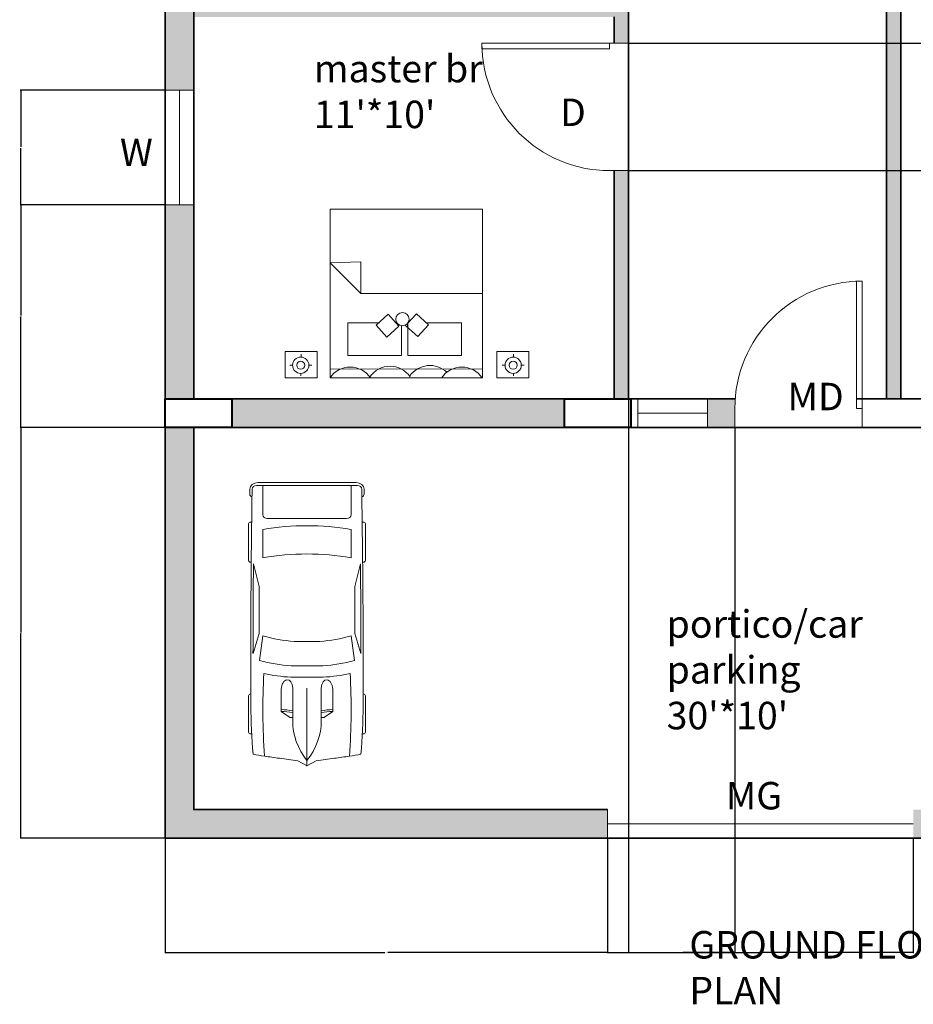
# Model space of a CAD drawing. Units: inches. Extents: x 1568 to 2529, y 2149 to 2897.
# Tile 1 of 16: x 1568 to 1849, y 2149 to 2459. Entities that reach past the tile are written whole.
import ezdxf

# ---------------------------------------------------------------- set-up
doc = ezdxf.new("R2010")
doc.units = ezdxf.units.IN
for name, color, linetype, lineweight in [('A-ANNO-DIMS', 2, 'Continuous', 18), ('A-AREA-IDEN', 210, 'Continuous', 18), ('A-COLS', 7, 'Continuous', 40), ('A-DOOR', 4, 'Continuous', 18), ('A-FURN', 8, 'Continuous', 18), ('A-WALL-PATT', 172, 'Continuous', 13), ('C-PKNG-VEHI', 8, 'Continuous', 13), ('text', 210, 'Continuous', 18), ('wall', 7, 'Continuous', 35), ('window', 130, 'Continuous', 18)]:
    doc.layers.add(name, color=color, linetype=linetype, lineweight=lineweight)
doc.styles.get("Standard").update_dxf_attribs({"font": 'arial.ttf'})
doc.dimstyles.get("Standard").update_dxf_attribs({"dimtxt": 0.18, "dimasz": 0.18, "dimexe": 0.18, "dimexo": 0.0625, "dimgap": 0.09, "dimtad": 0, "dimtih": 1, "dimtoh": 1, "dimdec": 4, "dimzin": 0, "dimdsep": 46, "dimtxsty": 'Standard', "dimcen": 0.09, "dimadec": 0, "dimazin": 0, "dimtfac": 1, "dimtdec": 4, "dimtofl": 0, "dimtmove": 0, "dimatfit": 3, "dimfxl": 1, "dimtolj": 1, "dimtzin": 0, "dimarcsym": 0})

# ---------------------------------------------------------------- blocks, each defined once
blk = doc.blocks.new('*U2')
for p, q in [((0, 0), (0, -6)), ((40, 0), (40, -6))]:
    blk.add_line(p, q)
blk.add_lwpolyline([(0, 0), (0, 40), (1.75, 40), (1.75, 0)], close=True)
blk.add_arc((0, 0), 40, 0, 90)
blk = doc.blocks.new('*U8')
for p, q in [((21.1, 37.41), (21.1, 36.83)), ((46.55, 38.89), (22.35, 38.89)), ((47.8, 37.39), (47.8, 37.41)), ((87.99, 31.87), (74.76, 35.92)), ((134.31, 35.6), (119.29, 31.78)), ((135.45, 37.07), (135.45, 37.41)), ((136.7, 38.89), (160.9, 38.89)), ((162.15, 37.41), (162.15, 36.77)), ((186.47, -33.5), (186.47, 33.5)), ((70.03, 31.54), (86.41, 29.35)), ((138.42, 29.35), (157.25, 29.35)), ((164.52, 26.39), (164.52, -26.39)), ((186.47, 29.35), (167.01, 29.35)), ((188.4, -32.76), (188.4, 32.76)), ((32.27, 11.63), (36.13, 17.17)), ((36.13, 17.17), (50.94, 17.17)), ((29.77, 9.51), (51.68, 9.51)), ((32.12, 9.51), (32.12, 11.15)), ((58.92, -10.77), (58.92, 10.77)), ((66.55, -10.53), (66.55, 10.53)), ((82.74, 8.5), (82.74, -8.5)), ((186.47, -10.53), (186.47, 10.53)), ((3.27, 6.13), (0.1, 0.41)), ((0, 0), (51.68, 0)), ((0.1, -0.41), (3.27, -6.13)), ((29.77, -9.51), (51.68, -9.51)), ((32.12, -9.51), (32.12, -11.15)), ((32.27, -11.63), (36.13, -17.17)), ((36.13, -17.17), (50.94, -17.17)), ((86.41, -29.35), (70.03, -31.54)), ((87.99, -31.87), (74.76, -35.92)), ((134.31, -35.6), (119.29, -31.78)), ((157.25, -29.35), (138.42, -29.35)), ((167.01, -29.35), (186.47, -29.35)), ((21.1, -37.41), (21.1, -36.83)), ((46.55, -38.89), (22.35, -38.89)), ((47.8, -37.39), (47.8, -37.41)), ((135.45, -37.07), (135.45, -37.41)), ((136.7, -38.89), (160.9, -38.89)), ((162.15, -37.41), (162.15, -36.77))]:
    blk.add_line(p, q)
for centre, major_axis, ratio, start_param, end_param in [((266.03, -27.52), (0, 313.31), 0.842304, 1.367076, 1.39176), ((41.19, -490.86), (0, 528.23), 0.842304, 0.00281, 0.075598), ((22.35, 37.41), (0, -1.48), 0.842304, 3.141593, 4.712389), ((64.48, -10555.62), (0, 10593.03), 0.842304, -0.013397, 0.002797), ((46.55, 37.41), (0, 1.48), 0.842304, -1.570796, 0), ((64.48, -10555.62), (0, -10591.55), 0.842304, 3.133765, 3.140441), ((136.7, 37.41), (0, -1.48), 0.842304, 3.141593, 4.712389), ((160.9, 37.41), (0, 1.48), 0.842304, -1.570796, 0), ((180.63, 35.84), (0, 2.22), 0.842304, -0.013017, 1.249894), ((64.48, -10556.36), (0, 10595.31), 0.842304, -0.013397, -0.013017), ((183.98, 33.5), (0, -2.96), 0.842304, 1.570796, 3.128196), ((183.98, 32.76), (0, -5.25), 0.842304, 1.570796, 3.128196), ((259.18, -27.52), (0, -305.3), 0.842304, 4.528606, 4.561838), ((37.47, -593.96), (0, -623.33), 0.842304, 3.096046, 3.200911), ((134.4, 5.39), (0, -89.78), 0.842304, 4.449482, 4.652344), ((135.29, 5.39), (0, 81.77), 0.842304, 1.245306, 1.50788), ((149.6, 2.8), (0, -79.58), 0.842304, 4.372215, 4.640744), ((95.79, -3666.35), (0, -3698.24), 0.842304, 3.134049, 3.144098), ((17.08, 0), (0, 147.02), 0.842304, 4.511394, 4.913384), ((35.91, 0), (0, 147.02), 0.842304, 4.511394, 4.913384), ((167.01, 26.39), (0, 2.96), 0.842304, 0, 1.570796), ((-204.49, 52.4), (0, -250.96), 0.842304, 1.385369, 1.434372), ((13.04, 17.01), (0, 27.42), 0.842304, 4.435146, 4.718221), ((14.2, 17.01), (0, 27.42), 0.842304, 4.435146, 4.718221), ((50.79, 13.34), (6.34, -0.36), 0.603834, -1.395552, 1.581315), ((29.77, -46.66), (0, 56.17), 0.842304, 0, 0.590319), ((32.75, 11.15), (0, 0.74), 0.842304, 0.879714, 1.570796), ((0.62, 0), (0, -0.74), 0.842304, 4.131459, 5.293319), ((-204.49, -52.4), (0, 250.96), 0.842304, -1.434372, -1.385369), ((29.77, 46.66), (0, 56.17), 0.842304, 2.551274, 3.141593), ((32.75, -11.15), (0, -0.74), 0.842304, 4.712389, 5.403472), ((13.04, -17.01), (0, -27.42), 0.842304, 1.564964, 1.848039), ((14.2, -17.01), (0, -27.42), 0.842304, 1.564964, 1.848039), ((134.4, -5.39), (0, -89.78), 0.842304, -1.510751, -1.307889), ((135.29, -5.39), (0, -81.77), 0.842304, -1.50788, -1.245306), ((149.6, -2.8), (0, -79.58), 0.842304, -1.499151, -1.230623), ((259.18, 27.52), (0, 305.3), 0.842304, 1.721348, 1.754579), ((266.03, 27.52), (0, 313.31), 0.842304, 1.749832, 1.774517), ((37.47, 593.96), (0, -623.33), 0.842304, -0.059319, 0.045547), ((95.79, 3666.35), (0, -3698.24), 0.842304, -0.002505, 0.007544), ((167.01, -26.39), (0, -2.96), 0.842304, 4.712389, 6.283185), ((183.98, -32.76), (0, -5.25), 0.842304, 0.013397, 1.570796), ((41.19, 490.86), (0, -528.23), 0.842304, -0.075598, -0.00281), ((22.35, -37.41), (0, 1.48), 0.842304, 1.570796, 3.141593), ((64.48, 10555.62), (0, 10593.03), 0.842304, 3.138796, 3.15499), ((46.55, -37.41), (0, -1.48), 0.842304, 0, 1.570796), ((64.48, 10555.62), (0, -10591.55), 0.842304, 0.001152, 0.007828), ((136.7, -37.41), (0, -1.48), 0.842304, -1.570796, 0), ((160.9, -37.41), (0, 1.48), 0.842304, 3.141593, 4.712389), ((180.63, -35.84), (0, -2.22), 0.842304, -1.249894, 0.013017), ((64.48, 10556.36), (0, 10595.31), 0.842304, 3.15461, 3.15499), ((183.98, -33.5), (0, 2.96), 0.842304, 3.15499, 4.712389)]:
    blk.add_ellipse(centre, major_axis=major_axis, ratio=ratio, start_param=start_param, end_param=end_param)
at = {"extrusion": (0, 0, -1)}
blk.add_ellipse((50.79, -13.34), major_axis=(6.34, 0.36), ratio=0.603834, start_param=-1.395552, end_param=1.581315, dxfattribs=at)
blk = doc.blocks.new('BED-WITH-NIGHTSTANDS')
for p, q in [((14.05, 36.12), (23.68, 36.4)), ((23.68, 26.45), (14.05, 36.12)), ((23.68, 36.4), (23.68, 26.45)), ((61.95, 26.45), (23.68, 26.45)), ((38.01, 16.14), (37.63, 16.49)), ((38.35, 15.84), (38.01, 16.14)), ((38.35, 16.98), (38.35, 15.84)), ((5, 6.48), (5, 7.42)), ((71.71, 6.48), (71.71, 7.42)), ((2.29, 3.95), (1.38, 3.95)), ((7.42, 3.92), (8.29, 3.92)), ((69, 3.95), (68.1, 3.95)), ((74.13, 3.92), (75, 3.92)), ((4.92, 1.35), (4.92, 0.55)), ((14.05, 2.79), (61.95, 2.73)), ((71.64, 1.35), (71.64, 0.55))]:
    blk.add_line(p, q)
for points in [[(14.05, 0), (61.95, 0), (61.95, 52.9), (14.05, 52.9)], [(31.9, 12.77), (35.7, 16.21), (32.32, 19.94), (28.52, 16.5)], [(10.04, 0), (0, 0), (0, 8.21), (10.04, 8.21)], [(76.49, 0), (66.44, 0), (66.44, 8.21), (76.49, 8.21)]]:
    blk.add_lwpolyline(points, close=True)
for points in [[(38.35, 16.98), (41.16, 20.08), (44.96, 16.64), (41.58, 12.91), (38.01, 16.14)], [(29.36, 17.26), (19.65, 17.26), (19.65, 6.93), (36.45, 6.93), (36.45, 16.34)], [(35.04, 17.26), (34.75, 17.26)], [(38.52, 17.23), (38.52, 6.93), (55.32, 6.93), (55.32, 17.26), (44.28, 17.26)], [(38.6, 17.26), (38.54, 17.26)]]:
    blk.add_lwpolyline(points)
for centre, radius in [((36.79, 18.4), 2.09), ((4.85, 3.92), 2.56), ((71.57, 3.92), 2.56), ((4.85, 3.92), 1.27), ((71.57, 3.92), 1.27)]:
    blk.add_circle(centre, radius)
for centre, start in [((20.4, -4.37), 34.5304), ((32.9, -4.09), 34.5304), ((45.42, -3.86), 46.3255), ((55.47, -4.37), 34.5304)]:
    blk.add_arc(centre, 7.71, start, 145.4696)
blk = doc.blocks.new('*D29')
at = {"layer": 'A-ANNO-DIMS', "color": 0, "lineweight": -2, "transparency": 16777216}
for p, q in [((1613.49, 2330.53), (1567.99, 2330.53)), ((1568.17, 2330.35), (1568.17, 2266.21)), ((1568.17, 2201.71), (1568.17, 2265.85)), ((1613.49, 2201.53), (1567.99, 2201.53))]:
    blk.add_line(p, q, dxfattribs=at)
at = {"layer": 'A-ANNO-DIMS', "color": 0, "transparency": 16777216}
for points in [[(1568.14, 2330.35), (1568.2, 2330.35), (1568.17, 2330.53)], [(1568.14, 2201.71), (1568.2, 2201.71), (1568.17, 2201.53)]]:
    blk.add_solid(points, dxfattribs=at)
at = {"layer": 'Defpoints', "color": 0, "transparency": 16777216}
for p in [(1568.17, 2330.53), (1613.55, 2330.53), (1613.55, 2201.53)]:
    blk.add_point(p, dxfattribs=at)
at = {"layer": 'A-ANNO-DIMS', "color": 0, "transparency": 16777216, "insert": (1568.17, 2266.03), "char_height": 0.18, "attachment_point": 5}
blk.add_mtext('\\A1;129', dxfattribs=at)
blk = doc.blocks.new('*D30')
at = {"layer": 'A-ANNO-DIMS', "color": 0, "lineweight": -2, "transparency": 16777216}
for p, q in [((1613.55, 2201.47), (1613.55, 2165.5)), ((1752.52, 2201.47), (1752.52, 2165.5)), ((1613.73, 2165.68), (1682.58, 2165.68)), ((1752.34, 2165.68), (1683.49, 2165.68))]:
    blk.add_line(p, q, dxfattribs=at)
at = {"layer": 'A-ANNO-DIMS', "color": 0, "transparency": 16777216}
for points in [[(1613.73, 2165.71), (1613.73, 2165.65), (1613.55, 2165.68)], [(1752.34, 2165.71), (1752.34, 2165.65), (1752.52, 2165.68)]]:
    blk.add_solid(points, dxfattribs=at)
at = {"layer": 'Defpoints', "color": 0, "transparency": 16777216}
for p in [(1613.55, 2201.53), (1752.52, 2201.53), (1752.52, 2165.68)]:
    blk.add_point(p, dxfattribs=at)
at = {"layer": 'A-ANNO-DIMS', "color": 0, "transparency": 16777216, "insert": (1683.03, 2165.68), "char_height": 0.18, "attachment_point": 5}
blk.add_mtext('\\A1;138.97', dxfattribs=at)
blk = doc.blocks.new('*D31')
at = {"layer": 'A-ANNO-DIMS', "color": 0, "lineweight": -2, "transparency": 16777216}
for p, q in [((1752.52, 2201.47), (1752.52, 2165.5)), ((1848.51, 2201.47), (1848.51, 2165.5)), ((1752.7, 2165.68), (1800.3, 2165.68)), ((1848.33, 2165.68), (1800.74, 2165.68))]:
    blk.add_line(p, q, dxfattribs=at)
at = {"layer": 'A-ANNO-DIMS', "color": 0, "transparency": 16777216}
for points in [[(1752.7, 2165.71), (1752.7, 2165.65), (1752.52, 2165.68)], [(1848.33, 2165.71), (1848.33, 2165.65), (1848.51, 2165.68)]]:
    blk.add_solid(points, dxfattribs=at)
at = {"layer": 'Defpoints', "color": 0, "transparency": 16777216}
for p in [(1752.52, 2201.53), (1848.51, 2201.53), (1848.51, 2165.68)]:
    blk.add_point(p, dxfattribs=at)
at = {"layer": 'A-ANNO-DIMS', "color": 0, "transparency": 16777216, "insert": (1800.52, 2165.68), "char_height": 0.18, "attachment_point": 5}
blk.add_mtext('\\A1;96', dxfattribs=at)
blk = doc.blocks.new('*D33')
at = {"layer": 'A-ANNO-DIMS', "color": 0, "lineweight": -2, "transparency": 16777216}
for p, q in [((1613.49, 2436.51), (1567.99, 2436.51)), ((1568.17, 2436.33), (1568.17, 2418.69)), ((1568.17, 2400.69), (1568.17, 2418.33)), ((1613.49, 2400.51), (1567.99, 2400.51))]:
    blk.add_line(p, q, dxfattribs=at)
at = {"layer": 'A-ANNO-DIMS', "color": 0, "transparency": 16777216}
for points in [[(1568.14, 2436.33), (1568.2, 2436.33), (1568.17, 2436.51)], [(1568.14, 2400.69), (1568.2, 2400.69), (1568.17, 2400.51)]]:
    blk.add_solid(points, dxfattribs=at)
at = {"layer": 'Defpoints', "color": 0, "transparency": 16777216}
for p in [(1568.17, 2436.51), (1613.55, 2436.51), (1613.55, 2400.51)]:
    blk.add_point(p, dxfattribs=at)
at = {"layer": 'A-ANNO-DIMS', "color": 0, "transparency": 16777216, "insert": (1568.17, 2418.51), "char_height": 0.18, "attachment_point": 5}
blk.add_mtext('\\A1;36', dxfattribs=at)
blk = doc.blocks.new('*D34')
at = {"layer": 'A-ANNO-DIMS', "color": 0, "lineweight": -2, "transparency": 16777216}
for p, q in [((1613.49, 2400.51), (1567.99, 2400.51)), ((1568.17, 2400.33), (1568.17, 2365.7)), ((1568.17, 2330.71), (1568.17, 2365.34)), ((1613.49, 2330.53), (1567.99, 2330.53))]:
    blk.add_line(p, q, dxfattribs=at)
at = {"layer": 'A-ANNO-DIMS', "color": 0, "transparency": 16777216}
for points in [[(1568.14, 2400.33), (1568.2, 2400.33), (1568.17, 2400.51)], [(1568.14, 2330.71), (1568.2, 2330.71), (1568.17, 2330.53)]]:
    blk.add_solid(points, dxfattribs=at)
at = {"layer": 'Defpoints', "color": 0, "transparency": 16777216}
for p in [(1568.17, 2400.51), (1613.55, 2400.51), (1613.55, 2330.53)]:
    blk.add_point(p, dxfattribs=at)
at = {"layer": 'A-ANNO-DIMS', "color": 0, "transparency": 16777216, "insert": (1568.17, 2365.52), "char_height": 0.18, "attachment_point": 5}
blk.add_mtext('\\A1;69.98', dxfattribs=at)
blk = doc.blocks.new('*D35')
at = {"layer": 'A-ANNO-DIMS', "color": 0, "lineweight": -2, "transparency": 16777216}
for p, q in [((1759.11, 2451.23), (2009.61, 2451.23)), ((2009.43, 2451.05), (2009.43, 2431.41)), ((2009.43, 2411.41), (2009.43, 2431.05)), ((1759.11, 2411.23), (2009.61, 2411.23))]:
    blk.add_line(p, q, dxfattribs=at)
at = {"layer": 'A-ANNO-DIMS', "color": 0, "transparency": 16777216}
for points in [[(2009.4, 2451.05), (2009.46, 2451.05), (2009.43, 2451.23)], [(2009.4, 2411.41), (2009.46, 2411.41), (2009.43, 2411.23)]]:
    blk.add_solid(points, dxfattribs=at)
at = {"layer": 'Defpoints', "color": 0, "transparency": 16777216}
for p in [(1759.05, 2451.23), (2009.43, 2451.23), (1759.05, 2411.23)]:
    blk.add_point(p, dxfattribs=at)
at = {"layer": 'A-ANNO-DIMS', "color": 0, "transparency": 16777216, "insert": (2009.43, 2431.23), "char_height": 0.18, "attachment_point": 5}
blk.add_mtext('\\A1;40', dxfattribs=at)
blk = doc.blocks.new('*D36')
at = {"layer": 'A-ANNO-DIMS', "color": 0, "lineweight": -2, "transparency": 16777216}
for p, q in [((1759.05, 2339.47), (1759.05, 2165.5)), ((1792.46, 2330.47), (1792.46, 2165.5)), ((1759.23, 2165.68), (1775.38, 2165.68)), ((1792.28, 2165.68), (1776.13, 2165.68))]:
    blk.add_line(p, q, dxfattribs=at)
at = {"layer": 'A-ANNO-DIMS', "color": 0, "transparency": 16777216}
for points in [[(1759.23, 2165.71), (1759.23, 2165.65), (1759.05, 2165.68)], [(1792.28, 2165.71), (1792.28, 2165.65), (1792.46, 2165.68)]]:
    blk.add_solid(points, dxfattribs=at)
at = {"layer": 'Defpoints', "color": 0, "transparency": 16777216}
for p in [(1759.05, 2339.53), (1792.46, 2330.53), (1792.46, 2165.68)]:
    blk.add_point(p, dxfattribs=at)
at = {"layer": 'A-ANNO-DIMS', "color": 0, "transparency": 16777216, "insert": (1775.76, 2165.68), "char_height": 0.18, "attachment_point": 5}
blk.add_mtext('\\A1;33.41', dxfattribs=at)

msp = doc.modelspace()

# ---------------------------------------------------------------- hatches: boundary and pattern name
at = {"layer": 'A-WALL-PATT'}
h = msp.add_hatch(color=256, dxfattribs=at)
h.dxf.hatch_style = 1
h.paths.add_polyline_path([(1738.1593, 2801.532), (1634.4841, 2801.532), (1634.4841, 2792.532), (1738.1593, 2792.532)])
h.paths.add_polyline_path([(1812.4114, 2801.532), (1759.0925, 2801.532), (1759.0925, 2792.532), (1812.4114, 2792.532)])
h.paths.add_polyline_path([(1952.647, 2801.532), (1848.4114, 2801.532), (1848.4114, 2792.532), (1952.647, 2792.532)])
h.paths.add_polyline_path([(1973.5509, 2792.532), (1964.5509, 2792.532), (1964.5509, 2699.1671), (1973.5509, 2699.1671)])
h.paths.add_polyline_path([(1973.5509, 2663.1671), (1964.5509, 2663.1671), (1964.5509, 2630.5978), (1973.5509, 2630.5978)])
h.paths.add_polyline_path([(1973.5509, 2609.6646), (1964.5509, 2609.6646), (1964.5509, 2572.3679), (1973.5509, 2572.3679)])
h.paths.add_polyline_path([(1622.5509, 2753.3576), (1622.3864, 2753.3576), (1613.5509, 2753.3576), (1613.5509, 2705.9172), (1622.5509, 2705.9172)])
h.paths.add_polyline_path([(1622.5509, 2669.9172), (1613.5509, 2669.9172), (1613.5509, 2624.532), (1622.5509, 2624.532)])
h.paths.add_polyline_path([(1759.0509, 2757.9833), (1754.5509, 2757.9833), (1754.5509, 2744.532), (1622.5509, 2744.532), (1622.5509, 2740.032), (1754.5509, 2740.032), (1754.5509, 2730.8156), (1759.0509, 2730.8156), (1759.0509, 2740.032)])
h.paths.add_polyline_path([(1759.0509, 2690.8156), (1754.5509, 2690.8156), (1754.5509, 2624.532), (1759.0509, 2624.532)])
h.paths.add_polyline_path([(1738.1177, 2620.032), (1634.4841, 2620.032), (1634.4841, 2615.532), (1738.1177, 2615.532)])
h.paths.add_polyline_path([(1622.5509, 2615.532), (1613.5509, 2615.532), (1613.5509, 2564.2764), (1622.5509, 2564.2764)])
h.paths.add_polyline_path([(1759.0509, 2411.2271), (1754.5509, 2411.2271), (1754.5509, 2339.532), (1759.0509, 2339.532)])
h.paths.add_polyline_path([(1759.0509, 2464.032), (1734.3925, 2464.032), (1622.5509, 2464.032), (1622.5509, 2459.532), (1736.5509, 2459.532), (1754.5509, 2459.532), (1754.5509, 2451.2271), (1759.0509, 2451.2271)])
h.paths.add_polyline_path([(1844.5509, 2471.532), (1858.1805, 2471.532), (1858.1805, 2476.032), (1844.5509, 2476.032), (1844.5509, 2510.0763), (1840.0509, 2510.0763), (1840.0509, 2476.032), (1840.0509, 2339.532), (1844.5509, 2339.532)])
h.paths.add_polyline_path([(1844.5509, 2596.032), (1964.5509, 2596.032), (1964.5509, 2600.532), (1840.0509, 2600.532), (1840.0509, 2570.0763), (1844.5509, 2570.0763)])
h.paths.add_polyline_path([(1964.5509, 2476.032), (1894.1805, 2476.032), (1894.1805, 2471.532), (1964.5509, 2471.532)])
h.paths.add_polyline_path([(1622.5509, 2528.2764), (1613.5509, 2528.2764), (1613.5509, 2436.512), (1622.5509, 2436.512)])
h.paths.add_polyline_path([(1622.5509, 2400.512), (1613.5509, 2400.512), (1613.5509, 2339.532), (1622.5509, 2339.532)])
h.paths.add_polyline_path([(1738.9144, 2339.532), (1634.4841, 2339.532), (1634.4841, 2330.532), (1738.9144, 2330.532)])
h.paths.add_polyline_path([(1792.463, 2336.532, -0.01876983), (1792.5756, 2339.532), (1783.8928, 2339.532), (1783.8928, 2330.532), (1792.463, 2330.532)])
h.paths.add_polyline_path([(1952.6177, 2339.532), (1885.2912, 2339.532), (1885.2912, 2330.532), (1952.6177, 2330.532)])
h.paths.add_polyline_path([(1973.5509, 2422.371), (1964.5509, 2422.371), (1964.5509, 2395.032), (1964.5509, 2387.286), (1964.5509, 2339.532), (1973.5509, 2339.532)])
h.paths.add_polyline_path([(1973.5509, 2536.3679), (1964.5509, 2536.3679), (1964.5509, 2476.032), (1964.5509, 2458.371), (1973.5509, 2458.371)])
h = msp.add_hatch(color=256, dxfattribs=at)
h.dxf.hatch_style = 1
h.paths.add_polyline_path([(1973.5509, 2330.532), (1964.5509, 2330.532), (1964.5509, 2210.532), (1848.5145, 2210.532), (1848.5145, 2201.532), (1973.5509, 2201.532)])
h.paths.add_polyline_path([(1622.5509, 2330.532), (1613.5509, 2330.532), (1613.5509, 2201.532), (1752.5179, 2201.532), (1752.5179, 2210.532), (1622.5509, 2210.532)])

# ---------------------------------------------------------------- linework, layer by layer
at = {"layer": 'A-COLS'}
for points in [[(1613.5509, 2339.532), (1634.4841, 2339.532), (1634.4841, 2330.532), (1613.5509, 2330.532)], [(1738.9144, 2339.532), (1759.8476, 2339.532), (1759.8476, 2330.532), (1738.9144, 2330.532)]]:
    msp.add_lwpolyline(points, close=True, dxfattribs=at)
at = {"layer": 'A-DOOR'}
for p, q in [((1752.5179, 2210.532), (1752.5179, 2201.532)), ((1752.5179, 2206.032), (1848.5145, 2206.032))]:
    msp.add_line(p, q, dxfattribs=at)
at = {"layer": 'wall'}
for p, q in [((1840.0509, 2339.532), (1840.0509, 2476.032)), ((1844.5509, 2339.532), (1844.5509, 2471.532)), ((1759.0509, 2339.532), (1759.0509, 2464.032)), ((1622.5509, 2459.532), (1622.5509, 2339.532)), ((1754.5509, 2451.2271), (1754.5509, 2459.532)), ((1754.5509, 2339.532), (1754.5509, 2411.2271)), ((1622.5509, 2339.532), (1754.5509, 2339.532)), ((1622.5509, 2339.532), (1792.5756, 2339.532)), ((1830.713, 2339.532), (1964.5509, 2339.532)), ((1622.5509, 2210.532), (1622.5509, 2330.532)), ((1622.5509, 2330.532), (1964.5509, 2330.532))]:
    msp.add_line(p, q, dxfattribs=at)
msp.add_lwpolyline([(1613.5509, 2201.532), (1973.5509, 2201.532), (1973.5509, 2801.532), (1613.5509, 2801.532)], close=True, dxfattribs=at)
for points in [[(1622.5509, 2615.532), (1622.5509, 2339.532)], [(1622.5509, 2330.532), (1622.5509, 2210.532), (1752.5179, 2210.532)]]:
    msp.add_lwpolyline(points, dxfattribs=at)
at = {"layer": 'window'}
for p, q in [((1613.5509, 2436.512), (1622.5509, 2436.512)), ((1618.0509, 2400.512), (1618.0509, 2436.512)), ((1613.5509, 2400.512), (1622.5509, 2400.512)), ((1761.9782, 2339.532), (1761.9782, 2330.532)), ((1783.8928, 2339.532), (1783.8928, 2330.532)), ((1761.9782, 2335.032), (1783.8928, 2335.032))]:
    msp.add_line(p, q, dxfattribs=at)

# ---------------------------------------------------------------- block references
at = {"layer": 'A-DOOR', "xscale": -1, "rotation": 90}
msp.add_blockref('*U2', (1753.0509, 2451.2271), dxfattribs=at)
at = {"layer": 'A-DOOR', "xscale": -1}
msp.add_blockref('*U2', (1832.463, 2336.532), dxfattribs=at)
at = {"layer": 'A-FURN'}
msp.add_blockref('BED-WITH-NIGHTSTANDS', (1651.277, 2346.1877), dxfattribs=at)
at = {"layer": 'C-PKNG-VEHI', "xscale": 0.4718531470838411, "yscale": 0.4718531470838411, "zscale": 0.4718531470838411, "rotation": 90}
msp.add_blockref('*U8', (1658.084, 2224.3358), dxfattribs=at)

# ---------------------------------------------------------------- texts
at = {"layer": 'A-AREA-IDEN', "attachment_point": 1}
for s, insert, char_height in [("master br\\P11'*10'", (1660.2444, 2447.5881), 8.62815), ("portico/car parking\\P30'*10'", (1771.0377, 2273.1556), 8.628146)]:
    msp.add_mtext_dynamic_manual_height_columns(s, width=94.297369, gutter_width=43.1407, heights=[0], dxfattribs=dict(at, insert=insert, char_height=char_height))
at = {"layer": 'text', "attachment_point": 1}
for s, heights, insert, char_height in [('D', [23.0437], (1737.5781, 2433.8598), 8.6281), ('W', [23.0437], (1599.3377, 2421.2711), 8.6281), ('MD', [23.0437], (1809.0166, 2344.6002), 8.62815), ('MG', [23.0437], (1789.622, 2219.2295), 8.62815), ('GROUND FLOOR PLAN', [0], (1778.1838, 2172.397), 8.628146)]:
    msp.add_mtext_dynamic_manual_height_columns(s, width=94.297369, gutter_width=43.1407, heights=heights, dxfattribs=dict(at, insert=insert, char_height=char_height))

# ---------------------------------------------------------------- dimensions: what is measured, and where the dimension line sits
at = {"layer": 'A-ANNO-DIMS'}
for base, p1, p2, override, picture, middle in [((2009.4302, 2451.2271), (1759.0509, 2411.2271), (1759.0509, 2451.2271), {"dimdec": 0, "dimlfac": 1, "dimrnd": 0, "dimzin": 0, "dimdsep": 46, "dimlunit": 2}, '*D35', (2009.4302, 2431.2271)), ((1568.1667, 2436.512), (1613.5509, 2400.512), (1613.5509, 2436.512), {"dimdec": 0, "dimlfac": 1, "dimrnd": 0, "dimzin": 0, "dimdsep": 46, "dimlunit": 2}, '*D33', (1568.1667, 2418.512)), ((1568.1667, 2400.512), (1613.5509, 2330.532), (1613.5509, 2400.512), {"dimdec": 2, "dimlfac": 1, "dimrnd": 0, "dimzin": 0, "dimdsep": 46, "dimlunit": 2}, '*D34', (1568.1667, 2365.522)), ((1568.1667, 2330.532), (1613.5509, 2201.532), (1613.5509, 2330.532), {"dimdec": 0, "dimlfac": 1, "dimrnd": 0, "dimzin": 0, "dimdsep": 46, "dimlunit": 2}, '*D29', (1568.1667, 2266.032))]:
    dim = msp.add_linear_dim(base=base, p1=p1, p2=p2, angle=90, dimstyle='Standard', override=override, dxfattribs=at)
    dim.commit()
    dim.dimension.update_dxf_attribs({"geometry": picture, "text_midpoint": middle})
for base, p1, p2, override, picture, middle in [((1792.463, 2165.682), (1759.0509, 2339.532), (1792.463, 2330.532), {"dimdec": 2, "dimlfac": 1, "dimrnd": 0, "dimzin": 0, "dimdsep": 46, "dimlunit": 2}, '*D36', (1775.7569, 2165.682)), ((1752.5179, 2165.682), (1613.5509, 2201.532), (1752.5179, 2201.532), {"dimdec": 2, "dimlfac": 1, "dimrnd": 0, "dimzin": 0, "dimdsep": 46, "dimlunit": 2}, '*D30', (1683.0344, 2165.682)), ((1848.5145, 2165.682), (1752.5179, 2201.532), (1848.5145, 2201.532), {"dimdec": 0, "dimlfac": 1, "dimrnd": 0, "dimzin": 0, "dimdsep": 46, "dimlunit": 2}, '*D31', (1800.5162, 2165.682))]:
    dim = msp.add_linear_dim(base=base, p1=p1, p2=p2, dimstyle='Standard', override=override, dxfattribs=at)
    dim.commit()
    dim.dimension.update_dxf_attribs({"geometry": picture, "text_midpoint": middle})

doc.saveas('drawing.dxf')
